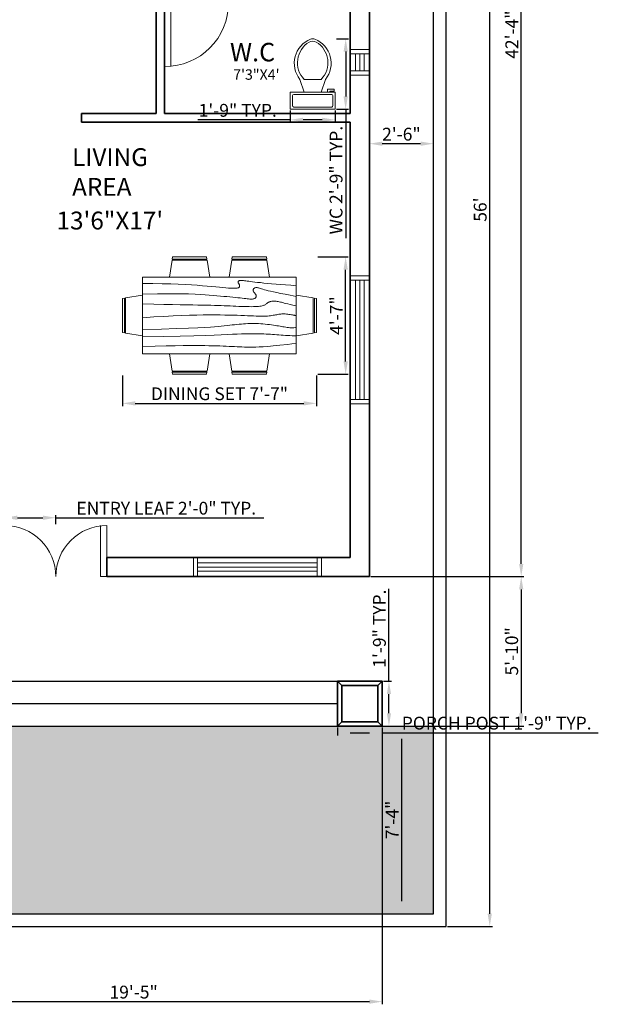
# Model space of a CAD drawing. Units: inches. Extents: x 104 to 647, y -91 to 674.
# Tile 2 of 3: x 376 to 647, y -91 to 371. Entities that reach past the tile are written whole.
import ezdxf

# ---------------------------------------------------------------- set-up
doc = ezdxf.new("R2010")
doc.units = ezdxf.units.IN
for name, color, linetype, lineweight in [('A-ANNO-DIMS', 2, 'Continuous', 18), ('A-AREA-IDEN', 7, 'Continuous', 18), ('A-COLS', 7, 'Continuous', 35), ('A-DOOR', 3, 'Continuous', 18), ('A-FLOR', 7, 'Continuous', 25), ('A-FLOR-FIXT', 9, 'Continuous', 18), ('A-FURN', 8, 'Continuous', 18), ('A-GLAZ', 4, 'Continuous', 18), ('A-WALL', 7, 'Continuous', 35), ('C-PROP', 7, 'Continuous', 25), ('L-PLNT-PATT', 3, 'Continuous', 13)]:
    doc.layers.add(name, color=color, linetype=linetype, lineweight=lineweight)
doc.styles.get("Standard").update_dxf_attribs({"font": 'arial.ttf'})
doc.dimstyles.new('ISO-25', dxfattribs={"dimtxt": 6, "dimasz": 6, "dimexe": 1.25, "dimexo": 0.625, "dimtad": 1, "dimdec": 1, "dimlunit": 3, "dimtxsty": 'Standard', "dimcen": 2.5, "dimadec": 0, "dimazin": 0, "dimtfac": 1, "dimtdec": 1, "dimtmove": 0, "dimatfit": 3, "dimfxl": 1, "dimarcsym": 0})

# ---------------------------------------------------------------- blocks, each defined once
blk = doc.blocks.new('Dining Set - 36 x 72 in.')
for p, q in [((-22.2343, 26.00059), (-23.4847, 17.99762)), ((-22.2304, 26), (-5.7608, 26)), ((-22, 27.5), (-22.1562, 26.50042)), ((-5.8416, 26.5), (-22.1534, 26.5)), ((-22, 27.5), (-6, 27.5)), ((-5.8437, 26.49966), (-6, 27.5)), ((-4.5152, 17.99762), (-5.7655, 25.99926)), ((5.7657, 26.00059), (4.5153, 17.99762)), ((5.7696, 26), (22.2392, 26)), ((6, 27.5), (5.8438, 26.50042)), ((22.1584, 26.5), (5.8466, 26.5)), ((6, 27.5), (22, 27.5)), ((22.1563, 26.49966), (22, 27.5)), ((23.4848, 17.99762), (22.2345, 25.99926)), ((36, 18), (-36, 18)), ((-36, 18), (-36, -18)), ((36, -18), (36, 18)), ((-44.0006, 8.23428), (-35.9976, 9.48474)), ((44.0006, 8.23428), (35.9976, 9.48474)), ((-45.5, 8), (-44.5004, 8.15617)), ((-45.5, 8), (-45.5, -8)), ((-44.5, -8.15843), (-44.5, 8.15338)), ((-44, 8.23041), (-44, -8.23915)), ((44, 8.23041), (44, -8.23915)), ((44.5, -8.15843), (44.5, 8.15338)), ((45.5, 8), (44.5005, 8.15617)), ((45.5, 8), (45.5, -8)), ((-44.4997, -8.15631), (-45.5, -8)), ((-35.9976, -9.48476), (-43.9993, -8.2345)), ((35.9976, -9.48476), (43.9993, -8.2345)), ((44.4997, -8.15631), (45.5, -8)), ((-36, -18), (36, -18)), ((-22.2343, -26.0006), (-23.4847, -17.99762)), ((-4.5152, -17.99762), (-5.7655, -25.99928)), ((5.7657, -26.0006), (4.5153, -17.99762)), ((23.4848, -17.99762), (22.2345, -25.99928)), ((-22.2304, -26), (-5.7608, -26)), ((-22, -27.5), (-22.1562, -26.50044)), ((-5.8416, -26.5), (-22.1534, -26.5)), ((-22, -27.5), (-6, -27.5)), ((-5.8437, -26.49967), (-6, -27.5)), ((5.7696, -26), (22.2392, -26)), ((6, -27.5), (5.8438, -26.50044)), ((22.1584, -26.5), (5.8466, -26.5)), ((6, -27.5), (22, -27.5)), ((22.1563, -26.49967), (22, -27.5))]:
    blk.add_line(p, q)
for points in [[(-36, 15), (-31.1772, 14.97754), (-26.8079, 14.91406), (-22.8538, 14.81543), (-19.276, 14.6875), (-16.0362, 14.53613), (-13.0957, 14.36718), (-10.4159, 14.18652), (-7.9583, 14), (-5.6904, 13.81315), (-3.6035, 13.63021), (-1.6954, 13.45508), (0.0365, 13.29166), (1.5945, 13.14388), (2.9811, 13.01562), (4.1988, 12.9108), (5.25, 12.83333), (6.1393, 12.78613), (6.8802, 12.76823), (7.4883, 12.77767), (7.9792, 12.8125), (8.3685, 12.87077), (8.6719, 12.95052), (8.9049, 13.0498), (9.0833, 13.16666), (9.2205, 13.29899), (9.3216, 13.44401), (9.3895, 13.59879), (9.4271, 13.76041), (9.4373, 13.92594), (9.4232, 14.09245), (9.3875, 14.257), (9.3333, 14.41666), (9.2638, 14.56917), (9.1836, 14.71484), (9.0975, 14.85465), (9.0104, 14.98958), (8.9272, 15.1206), (8.8529, 15.2487), (8.7922, 15.37483), (8.75, 15.5), (8.7305, 15.62467), (8.7344, 15.74739), (8.7617, 15.86621), (8.8125, 15.97916), (8.8867, 16.08431), (8.9844, 16.17968), (9.1055, 16.26334), (9.25, 16.33333), (9.4189, 16.38802), (9.6172, 16.42708), (9.8506, 16.45052), (10.125, 16.45833), (10.4463, 16.45052), (10.8203, 16.42708), (11.2529, 16.38802), (11.75, 16.33333), (12.3184, 16.26318), (12.9694, 16.17838), (13.7151, 16.07991), (14.5677, 15.96875), (15.5395, 15.84586), (16.6426, 15.71224), (17.8893, 15.56884), (19.2917, 15.41666), (20.859, 15.25667), (22.5879, 15.08984), (24.4721, 14.91715), (26.5052, 14.73958), (28.6809, 14.5581), (30.9929, 14.3737), (33.4347, 14.18733), (36, 14)], [(-36, 10), (-28.9766, 10.14274), (-23.1725, 10.20442), (-18.4241, 10.19775), (-14.5677, 10.13541), (-11.4399, 10.03011), (-8.877, 9.89453), (-6.7154, 9.74137), (-4.7917, 9.58333), (-2.9698, 9.43082), (-1.2246, 9.28515), (0.4415, 9.14534), (2.026, 9.01041), (3.5266, 8.87939), (4.9408, 8.7513), (6.266, 8.62516), (7.5, 8.5), (8.6411, 8.37549), (9.6914, 8.2539), (10.6538, 8.13818), (11.5312, 8.03125), (12.3267, 7.93603), (13.043, 7.85547), (13.6831, 7.79248), (14.25, 7.75), (14.7471, 7.7303), (15.1797, 7.73307), (15.5537, 7.75732), (15.875, 7.80208), (16.1494, 7.86637), (16.3828, 7.94922), (16.5811, 8.04964), (16.75, 8.16666), (16.8944, 8.29915), (17.0143, 8.44531), (17.1089, 8.60319), (17.1771, 8.77083), (17.218, 8.94629), (17.2305, 9.1276), (17.2137, 9.31282), (17.1667, 9.5), (17.0895, 9.6875), (16.987, 9.875), (16.8649, 10.0625), (16.7292, 10.25), (16.5856, 10.4375), (16.4401, 10.625), (16.2985, 10.8125), (16.1667, 11), (16.05, 11.18733), (15.9518, 11.3737), (15.8752, 11.5581), (15.8229, 11.73958), (15.798, 11.91715), (15.8034, 12.08984), (15.842, 12.25667), (15.9167, 12.41666), (16.0295, 12.56836), (16.1784, 12.70833), (16.3605, 12.83268), (16.5729, 12.9375), (16.8127, 13.01888), (17.0768, 13.07291), (17.3625, 13.0957), (17.6667, 13.08333), (17.9894, 13.03312), (18.3418, 12.94726), (18.7382, 12.82918), (19.1927, 12.68229), (19.7195, 12.51001), (20.3327, 12.31575), (21.0465, 12.10294), (21.875, 11.875), (22.8357, 11.63354), (23.959, 11.37304), (25.2786, 11.08618), (26.8282, 10.76562), (28.6414, 10.40405), (30.752, 9.99414), (33.1936, 9.52856), (36, 9)], [(-36, 5.5), (-30.7157, 5.3348), (-26.069, 5.20963), (-21.9946, 5.11767), (-18.4271, 5.05208), (-15.3009, 5.00602), (-12.5508, 4.97265), (-10.1112, 4.94515), (-7.9167, 4.91666), (-5.909, 4.88167), (-4.0586, 4.83984), (-2.3429, 4.79215), (-0.7396, 4.73958), (0.7739, 4.6831), (2.22, 4.6237), (3.6213, 4.56233), (5, 4.5), (6.373, 4.43782), (7.7344, 4.3776), (9.0723, 4.32129), (10.375, 4.27083), (11.6309, 4.22819), (12.8281, 4.19531), (13.9551, 4.17415), (15, 4.16666), (15.954, 4.17448), (16.819, 4.19791), (17.6001, 4.23698), (18.3021, 4.29166), (18.9299, 4.36198), (19.4883, 4.44791), (19.9823, 4.54948), (20.4167, 4.66666), (20.7969, 4.79899), (21.1302, 4.94401), (21.4245, 5.09879), (21.6875, 5.26041), (21.9271, 5.42594), (22.1511, 5.59245), (22.3672, 5.757), (22.5834, 5.91666), (22.8065, 6.06868), (23.0404, 6.21093), (23.2879, 6.34147), (23.5521, 6.45833), (23.8358, 6.55957), (24.142, 6.64323), (24.4735, 6.70735), (24.8334, 6.75), (25.2235, 6.76969), (25.642, 6.76692), (26.0858, 6.74267), (26.5521, 6.69791), (27.0379, 6.63362), (27.5404, 6.55078), (28.0565, 6.45036), (28.5834, 6.33333), (29.1242, 6.19987), (29.7071, 6.04687), (30.3661, 5.87044), (31.1354, 5.66666), (32.0493, 5.43164), (33.142, 5.16146), (34.4475, 4.85221), (36, 4.5)], [(-36, -1), (-30.7915, -0.6591), (-26.0195, -0.38216), (-21.6519, -0.16284), (-17.6563, 0.00521), (-14.0005, 0.12833), (-10.6523, 0.21289), (-7.5796, 0.26522), (-4.75, 0.29166), (-2.134, 0.29793), (0.2878, 0.28711), (2.5317, 0.26163), (4.6146, 0.22396), (6.5529, 0.17651), (8.3633, 0.12174), (10.0623, 0.06209), (11.6667, 0), (13.1899, -0.06201), (14.6341, -0.1211), (15.9982, -0.17432), (17.2813, -0.21875), (18.4823, -0.25147), (19.6003, -0.26953), (20.6343, -0.27002), (21.5834, -0.25), (22.4481, -0.20768), (23.2357, -0.14584), (23.9549, -0.06836), (24.6146, 0.02083), (25.2235, 0.11784), (25.7904, 0.21875), (26.3241, 0.31966), (26.8334, 0.41666), (27.3265, 0.50618), (27.8099, 0.58593), (28.2894, 0.65397), (28.7709, 0.70833), (29.2601, 0.74707), (29.763, 0.76823), (30.2855, 0.76985), (30.8334, 0.75), (31.4088, 0.70784), (31.9994, 0.64713), (32.589, 0.57275), (33.1615, 0.48958), (33.7008, 0.4025), (34.1908, 0.3164), (34.6153, 0.23616), (34.9584, 0.16666), (35.2099, 0.11165), (35.3848, 0.07031), (35.504, 0.04069), (35.5886, 0.02083), (35.6594, 0.00879), (35.7377, 0.0026), (35.8442, 0.00032), (36, 0)], [(-36, -6.5), (-27.1843, -6.31267), (-20.084, -6.1263), (-14.469, -5.9419), (-10.1094, -5.76042), (-6.7752, -5.58285), (-4.2363, -5.41016), (-2.2629, -5.24333), (-0.625, -5.08334), (0.8708, -4.93099), (2.2715, -4.78646), (3.5872, -4.64974), (4.8281, -4.52084), (6.0046, -4.39974), (7.127, -4.28646), (8.2053, -4.18099), (9.25, -4.08334), (10.2705, -3.99382), (11.2734, -3.91407), (12.2647, -3.84603), (13.25, -3.79167), (14.2354, -3.75293), (15.2266, -3.73177), (16.2295, -3.73015), (17.25, -3.75), (18.2912, -3.79248), (19.3451, -3.85547), (20.4009, -3.93604), (21.4479, -4.03125), (22.4754, -4.13819), (23.4727, -4.25391), (24.4289, -4.37549), (25.3334, -4.5), (26.1785, -4.62492), (26.9694, -4.74935), (27.7145, -4.87281), (28.4219, -4.99479), (29.1, -5.11483), (29.7572, -5.23242), (30.4016, -5.34709), (31.0417, -5.45834), (31.6837, -5.56437), (32.3262, -5.65821), (32.9658, -5.73153), (33.599, -5.77604), (34.2224, -5.78345), (34.8327, -5.74545), (35.4264, -5.65373), (36, -5.5)], [(-36, -10), (-26.4022, -9.81299), (-18.4675, -9.62891), (-11.9839, -9.45069), (-6.7396, -9.28125), (-2.5226, -9.12354), (0.8789, -8.98047), (3.6769, -8.85498), (6.0833, -8.75), (8.2767, -8.66765), (10.3021, -8.60677), (12.1712, -8.56543), (13.8958, -8.54167), (15.4876, -8.53353), (16.9583, -8.53907), (18.3197, -8.55632), (19.5834, -8.58334), (20.7616, -8.61841), (21.8685, -8.66081), (22.9188, -8.71004), (23.9271, -8.76563), (24.9081, -8.82707), (25.8763, -8.89388), (26.8465, -8.96558), (27.8334, -9.04167), (28.8474, -9.12118), (29.8828, -9.20117), (30.93, -9.27824), (31.9792, -9.34896), (33.0205, -9.40991), (34.0443, -9.45768), (35.0407, -9.48885), (36, -9.5)], [(-36, -14.5), (-30.0881, -14.33513), (-25.0332, -14.21224), (-20.7312, -14.12647), (-17.0781, -14.07292), (-13.97, -14.04671), (-11.3027, -14.04297), (-8.9724, -14.05681), (-6.875, -14.08334), (-4.9224, -14.11833), (-3.0905, -14.16016), (-1.3709, -14.20785), (0.2448, -14.26042), (1.7647, -14.3169), (3.1973, -14.3763), (4.5507, -14.43767), (5.8333, -14.5), (7.0554, -14.5621), (8.235, -14.62175), (9.3922, -14.67652), (10.5469, -14.72396), (11.7192, -14.76164), (12.929, -14.78711), (14.1965, -14.79794), (15.5417, -14.79167), (16.9933, -14.76424), (18.6152, -14.70508), (20.4804, -14.60197), (22.6615, -14.44271), (25.2312, -14.21509), (28.2624, -13.9069), (31.8277, -13.50594), (36, -13)]]:
    blk.add_lwpolyline(points)
blk = doc.blocks.new('Toilet - top')
for p, q in [((9.5, -6), (9.5, -2)), ((-10, -8.5), (-8, -8.5)), ((-10, -9.5), (-10, -8.5)), ((-8, -8.5), (-8, -8)), ((-7, -8), (-7, -9.5)), ((-4, -8), (-6, -14)), ((4, -8), (6, -14)), ((-7, -9.5), (-10, -9.5)), ((4, -14), (-4, -14))]:
    blk.add_line(p, q)
blk.add_lwpolyline([(10.5, -8), (10.5, 0), (-10.5, 0), (-10.5, -8)], close=True)
for points in [[(-9.5, -2), (-9.5, -6)], [(8.5, -1), (-8.5, -1)], [(-8.5, -7), (8.5, -7)]]:
    blk.add_lwpolyline(points)
for centre, radius, start, end in [((-8.62, -1.88), 0.884, 81.8699, 188.1301), ((8.62, -1.88), 0.884, 351.8699, 98.1301), ((-8.62, -6.12), 0.884, 171.8699, 278.1301), ((8.62, -6.12), 0.884, 261.8699, 8.1301), ((3.52, -21.58), 12.17, 141.4691, 247.9714), ((4.2, -21.82), 11.33, 136.3677, 238.9468), ((-3.52, -21.58), 12.17, 292.0284, 38.5307), ((-4.2, -21.82), 11.33, 301.053, 43.6321), ((0, -27.88), 4, 245.7318, 294.2682), ((0, -29), 4, 254.8605, 285.1395)]:
    blk.add_arc(centre, radius, start, end)
blk = doc.blocks.new('*D10')
at = {"layer": 'A-ANNO-DIMS', "color": 0, "lineweight": -2, "transparency": 16777216}
for p, q in [((539.79, 313.32), (539.79, 313.94)), ((569.79, 313.32), (569.79, 313.94)), ((563.79, 312.69), (545.79, 312.69))]:
    blk.add_line(p, q, dxfattribs=at)
at = {"layer": 'A-ANNO-DIMS', "color": 0, "transparency": 16777216}
for points in [[(545.79, 313.69), (545.79, 311.69), (539.79, 312.69)], [(563.79, 313.69), (563.79, 311.69), (569.79, 312.69)]]:
    blk.add_solid(points, dxfattribs=at)
at = {"layer": 'Defpoints', "color": 0, "transparency": 16777216}
for p in [(539.79, 312.69), (539.79, 312.69), (569.79, 312.69)]:
    blk.add_point(p, dxfattribs=at)
at = {"layer": 'A-ANNO-DIMS', "color": 0, "transparency": 16777216, "insert": (554.79, 316.38), "char_height": 6, "attachment_point": 5}
blk.add_mtext('2\'-6"', dxfattribs=at)
blk = doc.blocks.new('*D12')
at = {"layer": 'A-ANNO-DIMS', "color": 0, "lineweight": -2, "transparency": 16777216}
for p, q in [((576.41, 617.8), (597.43, 617.8)), ((596.18, -48.2), (596.18, 611.8)), ((576.41, -54.2), (597.43, -54.2))]:
    blk.add_line(p, q, dxfattribs=at)
at = {"layer": 'A-ANNO-DIMS', "color": 0, "transparency": 16777216}
for points in [[(595.18, 611.8), (597.18, 611.8), (596.18, 617.8)], [(595.18, -48.2), (597.18, -48.2), (596.18, -54.2)]]:
    blk.add_solid(points, dxfattribs=at)
at = {"layer": 'Defpoints', "color": 0, "transparency": 16777216}
for p in [(575.79, 617.8), (596.18, 617.8), (575.79, -54.2)]:
    blk.add_point(p, dxfattribs=at)
at = {"layer": 'A-ANNO-DIMS', "color": 0, "transparency": 16777216, "insert": (592.49, 281.8), "char_height": 6, "attachment_point": 5, "rotation": 90}
blk.add_mtext("56'", dxfattribs=at)
blk = doc.blocks.new('*D14')
at = {"layer": 'A-ANNO-DIMS', "color": 0, "lineweight": -2, "transparency": 16777216}
for p, q in [((535.91, 39.8), (556.1, 39.8)), ((554.85, 33.8), (554.85, -42.2)), ((546.41, -48.2), (556.1, -48.2))]:
    blk.add_line(p, q, dxfattribs=at)
at = {"layer": 'A-ANNO-DIMS', "color": 0, "transparency": 16777216}
for points in [[(553.85, 33.8), (555.85, 33.8), (554.85, 39.8)], [(553.85, -42.2), (555.85, -42.2), (554.85, -48.2)]]:
    blk.add_solid(points, dxfattribs=at)
at = {"layer": 'Defpoints', "color": 0, "transparency": 16777216}
for p in [(535.29, 39.8), (545.79, -48.2), (554.85, -48.2)]:
    blk.add_point(p, dxfattribs=at)
at = {"layer": 'A-ANNO-DIMS', "color": 0, "transparency": 16777216, "insert": (551.23, -4.2), "char_height": 6, "attachment_point": 5, "rotation": 90}
blk.add_mtext('7\'-4"', dxfattribs=at)
blk = doc.blocks.new('WIN-60IN')
for p, q in [((60, 9), (0, 9)), ((0, 9), (0, 0)), ((2, 9), (2, 0)), ((2, 6.5), (58, 6.5)), ((58, 0), (58, 9)), ((60, 0), (60, 9)), ((0, 0), (60, 0)), ((2, 4.5), (58, 4.5)), ((2, 2.5), (58, 2.5))]:
    blk.add_line(p, q)
blk = doc.blocks.new('WIN-12IN')
for p, q in [((12, 9), (0, 9)), ((0, 9), (0, 0)), ((2, 9), (2, 0)), ((2, 6.5), (10, 6.5)), ((10, 0), (10, 9)), ((12, 0), (12, 9)), ((0, 0), (12, 0)), ((2, 4.5), (10, 4.5)), ((2, 2.5), (10, 2.5))]:
    blk.add_line(p, q)
blk = doc.blocks.new('DOOR-SWING-30IN')
for p, q in [((0, 0), (0, 30)), ((0, 30), (3, 30)), ((3, 0), (3, 30))]:
    blk.add_line(p, q)
blk.add_arc((0, 30), 30, 270, 0)
blk = doc.blocks.new('DOOR-ENTRY-LEAF-24IN')
for p, q in [((0, 24), (0, 0)), ((3, 24), (3, 0)), ((0, 0), (3, 0))]:
    blk.add_line(p, q)
blk.add_arc((0, 0), 24, 0, 90)
blk = doc.blocks.new('POST-21IN')
for p, q in [((0, 21), (2, 19)), ((19, 19), (21, 21)), ((0, 0), (2, 2)), ((19, 2), (21, 0))]:
    blk.add_line(p, q)
for points in [[(0, 0), (21, 0), (21, 21), (0, 21)], [(2, 2), (19, 2), (19, 19), (2, 19)]]:
    blk.add_lwpolyline(points, close=True)
blk = doc.blocks.new('*D25')
at = {"layer": 'A-ANNO-DIMS', "color": 0, "lineweight": -2, "transparency": 16777216}
for p, q in [((524.32, 361.86), (529.91, 361.86)), ((528.66, 355.86), (528.66, 334.81)), ((524.32, 328.81), (529.91, 328.81)), ((528.66, 328.81), (528.66, 268.45))]:
    blk.add_line(p, q, dxfattribs=at)
at = {"layer": 'A-ANNO-DIMS', "color": 0, "transparency": 16777216}
for points in [[(527.66, 355.86), (529.66, 355.86), (528.66, 361.86)], [(527.66, 334.81), (529.66, 334.81), (528.66, 328.81)]]:
    blk.add_solid(points, dxfattribs=at)
at = {"layer": 'Defpoints', "color": 0, "transparency": 16777216}
for p in [(523.7, 361.86), (523.7, 328.81), (528.66, 328.81)]:
    blk.add_point(p, dxfattribs=at)
at = {"layer": 'A-ANNO-DIMS', "color": 0, "transparency": 16777216, "insert": (524.93, 295.63), "char_height": 6, "attachment_point": 5, "rotation": 90}
blk.add_mtext('WC 2\'-9" TYP.', dxfattribs=at)
blk = doc.blocks.new('*D26')
at = {"layer": 'A-ANNO-DIMS', "color": 0, "lineweight": -2, "transparency": 16777216}
for p, q in [((502.7, 328.19), (502.7, 322.61)), ((523.7, 328.19), (523.7, 322.61)), ((502.7, 323.86), (459.44, 323.86)), ((517.7, 323.86), (508.7, 323.86))]:
    blk.add_line(p, q, dxfattribs=at)
at = {"layer": 'A-ANNO-DIMS', "color": 0, "transparency": 16777216}
for points in [[(508.7, 324.86), (508.7, 322.86), (502.7, 323.86)], [(517.7, 324.86), (517.7, 322.86), (523.7, 323.86)]]:
    blk.add_solid(points, dxfattribs=at)
at = {"layer": 'Defpoints', "color": 0, "transparency": 16777216}
for p in [(502.7, 328.81), (523.7, 328.81), (502.7, 323.86)]:
    blk.add_point(p, dxfattribs=at)
at = {"layer": 'A-ANNO-DIMS', "color": 0, "transparency": 16777216, "insert": (478.07, 327.55), "char_height": 6, "attachment_point": 5}
blk.add_mtext('1\'-9" TYP.', dxfattribs=at)
blk = doc.blocks.new('*D35')
at = {"layer": 'A-ANNO-DIMS', "color": 0, "lineweight": -2, "transparency": 16777216}
for p, q in [((368.79, 134.42), (368.79, 138.65)), ((392.79, 134.42), (392.79, 138.65)), ((374.79, 137.4), (386.79, 137.4)), ((392.79, 137.4), (490.32, 137.4))]:
    blk.add_line(p, q, dxfattribs=at)
at = {"layer": 'A-ANNO-DIMS', "color": 0, "transparency": 16777216}
for points in [[(374.79, 138.4), (374.79, 136.4), (368.79, 137.4)], [(386.79, 138.4), (386.79, 136.4), (392.79, 137.4)]]:
    blk.add_solid(points, dxfattribs=at)
at = {"layer": 'Defpoints', "color": 0, "transparency": 16777216}
for p in [(392.79, 137.4), (368.79, 133.8), (392.79, 133.8)]:
    blk.add_point(p, dxfattribs=at)
at = {"layer": 'A-ANNO-DIMS', "color": 0, "transparency": 16777216, "insert": (444.56, 141.09), "char_height": 6, "attachment_point": 5}
blk.add_mtext('ENTRY LEAF 2\'-0" TYP.', dxfattribs=at)
blk = doc.blocks.new('*D37')
at = {"layer": 'A-ANNO-DIMS', "color": 0, "lineweight": -2, "transparency": 16777216}
for p, q in [((524.79, 39.17), (524.79, 35.4)), ((545.79, 39.17), (545.79, 35.4)), ((530.79, 36.65), (539.79, 36.65)), ((545.79, 36.65), (647.06, 36.65))]:
    blk.add_line(p, q, dxfattribs=at)
at = {"layer": 'A-ANNO-DIMS', "color": 0, "transparency": 16777216}
for points in [[(530.79, 37.65), (530.79, 35.65), (524.79, 36.65)], [(539.79, 37.65), (539.79, 35.65), (545.79, 36.65)]]:
    blk.add_solid(points, dxfattribs=at)
at = {"layer": 'Defpoints', "color": 0, "transparency": 16777216}
for p in [(524.79, 39.8), (545.79, 39.8), (545.79, 36.65)]:
    blk.add_point(p, dxfattribs=at)
at = {"layer": 'A-ANNO-DIMS', "color": 0, "transparency": 16777216, "insert": (599.43, 40.38), "char_height": 6, "attachment_point": 5}
blk.add_mtext('PORCH POST 1\'-9" TYP.', dxfattribs=at)
blk = doc.blocks.new('*D38')
at = {"layer": 'A-ANNO-DIMS', "color": 0, "lineweight": -2, "transparency": 16777216}
for p, q in [((548.94, 60.8), (548.94, 104.06)), ((546.41, 60.8), (550.19, 60.8)), ((548.94, 45.8), (548.94, 54.8)), ((546.41, 39.8), (550.19, 39.8))]:
    blk.add_line(p, q, dxfattribs=at)
at = {"layer": 'A-ANNO-DIMS', "color": 0, "transparency": 16777216}
for points in [[(547.94, 54.8), (549.94, 54.8), (548.94, 60.8)], [(547.94, 45.8), (549.94, 45.8), (548.94, 39.8)]]:
    blk.add_solid(points, dxfattribs=at)
at = {"layer": 'Defpoints', "color": 0, "transparency": 16777216}
for p in [(545.79, 60.8), (548.94, 60.8), (545.79, 39.8)]:
    blk.add_point(p, dxfattribs=at)
at = {"layer": 'A-ANNO-DIMS', "color": 0, "transparency": 16777216, "insert": (545.25, 85.43), "char_height": 6, "attachment_point": 5, "rotation": 90}
blk.add_mtext('1\'-9" TYP.', dxfattribs=at)
blk = doc.blocks.new('*D39')
at = {"layer": 'A-ANNO-DIMS', "color": 0, "lineweight": -2, "transparency": 16777216}
for p, q in [((424, 204.03), (424, 189.75)), ((515, 204.03), (515, 189.75)), ((430, 191), (509, 191))]:
    blk.add_line(p, q, dxfattribs=at)
at = {"layer": 'A-ANNO-DIMS', "color": 0, "transparency": 16777216}
for points in [[(430, 192), (430, 190), (424, 191)], [(509, 192), (509, 190), (515, 191)]]:
    blk.add_solid(points, dxfattribs=at)
at = {"layer": 'Defpoints', "color": 0, "transparency": 16777216}
for p in [(424, 204.65), (515, 204.65), (515, 191)]:
    blk.add_point(p, dxfattribs=at)
at = {"layer": 'A-ANNO-DIMS', "color": 0, "transparency": 16777216, "insert": (469.5, 194.73), "char_height": 6, "attachment_point": 5}
blk.add_mtext('DINING SET 7\'-7"', dxfattribs=at)
blk = doc.blocks.new('*D40')
at = {"layer": 'A-ANNO-DIMS', "color": 0, "lineweight": -2, "transparency": 16777216}
for p, q in [((515.62, 259.65), (529.9, 259.65)), ((528.65, 210.65), (528.65, 253.65)), ((515.62, 204.65), (529.9, 204.65))]:
    blk.add_line(p, q, dxfattribs=at)
at = {"layer": 'A-ANNO-DIMS', "color": 0, "transparency": 16777216}
for points in [[(527.65, 253.65), (529.65, 253.65), (528.65, 259.65)], [(527.65, 210.65), (529.65, 210.65), (528.65, 204.65)]]:
    blk.add_solid(points, dxfattribs=at)
at = {"layer": 'Defpoints', "color": 0, "transparency": 16777216}
for p in [(515, 259.65), (528.65, 259.65), (515, 204.65)]:
    blk.add_point(p, dxfattribs=at)
at = {"layer": 'A-ANNO-DIMS', "color": 0, "transparency": 16777216, "insert": (525.02, 232.15), "char_height": 6, "attachment_point": 5, "rotation": 90}
blk.add_mtext('4\'-7"', dxfattribs=at)
blk = doc.blocks.new('*D52')
at = {"layer": 'A-ANNO-DIMS', "color": 0, "lineweight": -2, "transparency": 16777216}
for p, q in [((540.41, 617.8), (612.19, 617.8)), ((610.94, 115.8), (610.94, 611.8)), ((540.41, 109.8), (612.19, 109.8))]:
    blk.add_line(p, q, dxfattribs=at)
at = {"layer": 'A-ANNO-DIMS', "color": 0, "transparency": 16777216}
for points in [[(609.94, 611.8), (611.94, 611.8), (610.94, 617.8)], [(609.94, 115.8), (611.94, 115.8), (610.94, 109.8)]]:
    blk.add_solid(points, dxfattribs=at)
at = {"layer": 'Defpoints', "color": 0, "transparency": 16777216}
for p in [(539.79, 617.8), (610.94, 617.8), (539.79, 109.8)]:
    blk.add_point(p, dxfattribs=at)
at = {"layer": 'A-ANNO-DIMS', "color": 0, "transparency": 16777216, "insert": (607.3, 363.8), "char_height": 6, "attachment_point": 5, "rotation": 90}
blk.add_mtext('42\'-4"', dxfattribs=at)
blk = doc.blocks.new('*D53')
at = {"layer": 'A-ANNO-DIMS', "color": 0, "lineweight": -2, "transparency": 16777216}
for p, q in [((312.79, 39.17), (312.79, -90.6)), ((545.79, 39.17), (545.79, -90.6)), ((318.79, -89.35), (539.79, -89.35))]:
    blk.add_line(p, q, dxfattribs=at)
at = {"layer": 'A-ANNO-DIMS', "color": 0, "transparency": 16777216}
for points in [[(318.79, -88.35), (318.79, -90.35), (312.79, -89.35)], [(539.79, -88.35), (539.79, -90.35), (545.79, -89.35)]]:
    blk.add_solid(points, dxfattribs=at)
at = {"layer": 'Defpoints', "color": 0, "transparency": 16777216}
for p in [(312.79, 39.8), (545.79, 39.8), (545.79, -89.35)]:
    blk.add_point(p, dxfattribs=at)
at = {"layer": 'A-ANNO-DIMS', "color": 0, "transparency": 16777216, "insert": (429.29, -85.66), "char_height": 6, "attachment_point": 5}
blk.add_mtext('19\'-5"', dxfattribs=at)
blk = doc.blocks.new('*D54')
at = {"layer": 'A-ANNO-DIMS', "color": 0, "lineweight": -2, "transparency": 16777216}
for p, q in [((540.41, 109.8), (612.19, 109.8)), ((610.94, 103.8), (610.94, 45.8)), ((546.41, 39.8), (612.19, 39.8))]:
    blk.add_line(p, q, dxfattribs=at)
at = {"layer": 'A-ANNO-DIMS', "color": 0, "transparency": 16777216}
for points in [[(609.94, 103.8), (611.94, 103.8), (610.94, 109.8)], [(609.94, 45.8), (611.94, 45.8), (610.94, 39.8)]]:
    blk.add_solid(points, dxfattribs=at)
at = {"layer": 'Defpoints', "color": 0, "transparency": 16777216}
for p in [(539.79, 109.8), (545.79, 39.8), (610.94, 39.8)]:
    blk.add_point(p, dxfattribs=at)
at = {"layer": 'A-ANNO-DIMS', "color": 0, "transparency": 16777216, "insert": (607.25, 74.8), "char_height": 6, "attachment_point": 5, "rotation": 90}
blk.add_mtext('5\'-10"', dxfattribs=at)

msp = doc.modelspace()

# ---------------------------------------------------------------- hatches: boundary and pattern name
at = {"layer": 'L-PLNT-PATT'}
h = msp.add_hatch(dxfattribs=at)
h.set_pattern_fill('GRASS', color=256, scale=0.2)
h.paths.add_polyline_path([(569.79, 39.8), (546.01, 39.8), (524.79, 39.8), (312.79, 39.8), (157.79, 39.8), (157.79, -48.2), (205.79, -48.2), (545.79, -48.2), (569.79, -48.2)])

# ---------------------------------------------------------------- linework, layer by layer
at = {"layer": 'A-FLOR'}
for p, q in [((312.79, 60.8), (545.79, 60.8)), ((333.79, 50.3), (524.79, 50.3)), ((312.79, 39.8), (545.79, 39.8))]:
    msp.add_line(p, q, dxfattribs=at)
at = {"layer": 'A-WALL'}
for p, q in [((539.79, 109.8), (539.79, 608.8)), ((439.79, 326.8), (439.79, 378.8)), ((443.79, 326.8), (443.79, 378.8)), ((530.79, 326.8), (530.79, 374.8)), ((439.79, 326.8), (404.79, 326.8)), ((404.79, 326.8), (404.79, 322.8)), ((530.79, 326.8), (443.79, 326.8)), ((439.79, 322.8), (404.79, 322.8)), ((439.79, 322.8), (443.79, 322.8)), ((530.79, 322.8), (443.79, 322.8)), ((530.79, 118.8), (530.79, 322.8)), ((439.79, 118.8), (416.79, 118.8)), ((416.79, 118.8), (416.79, 109.8)), ((439.79, 118.8), (443.79, 118.8)), ((530.79, 118.8), (443.79, 118.8)), ((439.79, 109.8), (416.79, 109.8)), ((439.79, 109.8), (443.79, 109.8)), ((539.79, 109.8), (443.79, 109.8))]:
    msp.add_line(p, q, dxfattribs=at)
at = {"layer": 'C-PROP'}
for p, q in [((575.79, -54.2), (575.79, 617.8)), ((569.79, -48.2), (569.79, 608.8)), ((205.79, -48.2), (545.79, -48.2)), ((545.79, -48.2), (569.79, -48.2)), ((205.79, -54.2), (545.79, -54.2)), ((545.79, -54.2), (575.79, -54.2))]:
    msp.add_line(p, q, dxfattribs=at)

# ---------------------------------------------------------------- block references
at = {"layer": 'A-COLS'}
msp.add_blockref('POST-21IN', (524.79, 39.8), dxfattribs=at)
at = {"layer": 'A-DOOR'}
for name, p in [('DOOR-SWING-30IN', (443.79, 348.8)), ('DOOR-ENTRY-LEAF-24IN', (368.79, 109.8))]:
    msp.add_blockref(name, p, dxfattribs=at)
at = {"layer": 'A-DOOR', "extrusion": (0, 0, -1), "zscale": -1}
msp.add_blockref('DOOR-ENTRY-LEAF-24IN', (-416.79, 109.8), dxfattribs=at)
at = {"layer": 'A-FLOR-FIXT', "rotation": 180}
msp.add_blockref('Toilet - top', (513.2, 328.81), dxfattribs=at)
at = {"layer": 'A-FURN'}
msp.add_blockref('Dining Set - 36 x 72 in.', (469.5, 232.15), dxfattribs=at)
at = {"layer": 'A-GLAZ'}
for name, p, rotation in [('WIN-12IN', (530.79, 356.8), 269.9999999999999), ('WIN-60IN', (539.79, 190.8), 90.00000000000006)]:
    msp.add_blockref(name, p, dxfattribs=dict(at, rotation=rotation))
msp.add_blockref('WIN-60IN', (457.29, 109.8), dxfattribs=at)

# ---------------------------------------------------------------- texts
at = {"layer": 'A-AREA-IDEN', "attachment_point": 1}
for s, width, gutter_width, insert, char_height in [('W.C', 233.519, 43.29, (474.43, 359.93), 8.657), ('7\'3"X4\'', 131.4694, 24.37, (475.93, 347.53), 4.874), ('LIVING\\PAREA', 225.5639, 41.81, (400.45, 310.57), 8.362), ('13\'6"X17\'', 225.5639, 41.81, (393.15, 280.86), 8.362)]:
    msp.add_mtext_dynamic_manual_height_columns(s, width=width, gutter_width=gutter_width, heights=[0], dxfattribs=dict(at, insert=insert, char_height=char_height))

# ---------------------------------------------------------------- dimensions: what is measured, and where the dimension line sits
at = {"layer": 'A-ANNO-DIMS'}
for base, p1, p2, angle, override, picture, middle in [((610.94, 617.8), (539.79, 109.8), (539.79, 617.8), 90, {"dimdec": 1, "dimlfac": 1, "dimrnd": 0, "dimzin": 1, "dimdsep": 46, "dimlunit": 4, "dimfrac": 2}, '*D52', (607.3, 363.8)), ((539.79, 312.69), (569.79, 312.69), (539.79, 312.69), 180, {"dimclrd": 0, "dimclre": 0, "dimclrt": 0}, '*D10', (554.79, 316.38)), ((528.65, 259.65), (515, 204.65), (515, 259.65), 90, {"dimdec": 1, "dimlfac": 1, "dimrnd": 0, "dimzin": 1, "dimdsep": 46, "dimlunit": 4, "dimfrac": 2}, '*D40', (525.02, 232.15)), ((610.94, 39.8), (539.79, 109.8), (545.79, 39.8), 90, {"dimdec": 1, "dimlfac": 1, "dimrnd": 0, "dimzin": 1, "dimdsep": 46, "dimlunit": 4, "dimfrac": 2}, '*D54', (607.25, 74.8)), ((554.85, -48.2), (535.29, 39.8), (545.79, -48.2), 90, {"dimclrd": 0, "dimclre": 0, "dimclrt": 0}, '*D14', (551.23, -4.2))]:
    dim = msp.add_linear_dim(base=base, p1=p1, p2=p2, angle=angle, dimstyle='ISO-25', override=override, dxfattribs=at)
    dim.commit()
    dim.dimension.update_dxf_attribs({"geometry": picture, "text_midpoint": middle})
dim = msp.add_aligned_dim(p1=(575.79, -54.2), p2=(575.79, 617.8), distance=-20.39, dimstyle='ISO-25', override={"dimclrd": 0, "dimclre": 0, "dimclrt": 0}, dxfattribs=at)
dim.commit()
dim.dimension.update_dxf_attribs({"geometry": '*D12', "text_midpoint": (592.49, 281.8)})
for base, p1, p2, angle, text, picture, middle in [((528.6561, 328.8148), (523.6992, 361.861), (523.6992, 328.8148), 270, 'WC <> TYP.', '*D25', (524.9288, 295.6339)), ((502.7, 323.86), (523.7, 328.81), (502.7, 328.81), 180, '<> TYP.', '*D26', (478.07, 327.55)), ((548.94, 60.8), (545.79, 39.8), (545.79, 60.8), 90, '<> TYP.', '*D38', (545.25, 85.43))]:
    dim = msp.add_linear_dim(base=base, p1=p1, p2=p2, angle=angle, text=text, dimstyle='ISO-25', override={"dimdec": 1, "dimlfac": 1, "dimrnd": 0, "dimzin": 1, "dimdsep": 46, "dimlunit": 4, "dimfrac": 2}, dxfattribs=at)
    dim.commit()
    dim.dimension.update_dxf_attribs({"geometry": picture, "text_midpoint": middle})
for base, p1, p2, text, picture, middle in [((515, 191), (424, 204.65), (515, 204.65), 'DINING SET <>', '*D39', (469.5, 194.73)), ((392.79, 137.4), (368.79, 133.8), (392.79, 133.8), 'ENTRY LEAF <> TYP.', '*D35', (444.56, 141.09)), ((545.79, 36.65), (524.79, 39.8), (545.79, 39.8), 'PORCH POST <> TYP.', '*D37', (599.43, 40.38))]:
    dim = msp.add_linear_dim(base=base, p1=p1, p2=p2, text=text, dimstyle='ISO-25', override={"dimdec": 1, "dimlfac": 1, "dimrnd": 0, "dimzin": 1, "dimdsep": 46, "dimlunit": 4, "dimfrac": 2}, dxfattribs=at)
    dim.commit()
    dim.dimension.update_dxf_attribs({"geometry": picture, "text_midpoint": middle})
dim = msp.add_linear_dim(base=(545.79, -89.35), p1=(312.79, 39.8), p2=(545.79, 39.8), dimstyle='ISO-25', override={"dimdec": 1, "dimlfac": 1, "dimrnd": 0, "dimzin": 1, "dimdsep": 46, "dimlunit": 4, "dimfrac": 2}, dxfattribs=at)
dim.commit()
dim.dimension.update_dxf_attribs({"geometry": '*D53', "text_midpoint": (429.29, -85.66)})

doc.saveas('drawing.dxf')
